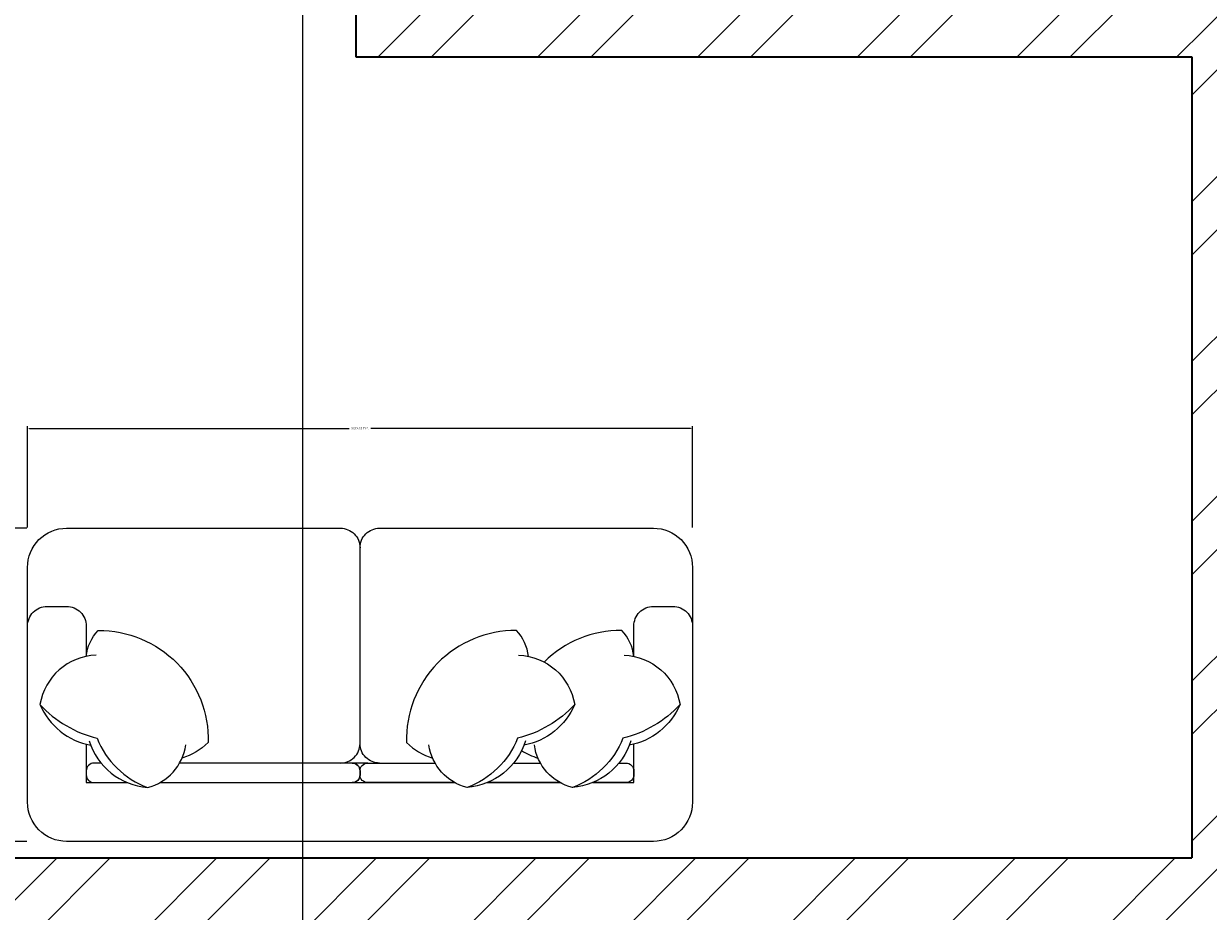
# Model space of a CAD drawing. Units: inches. Extents: x 2552 to 3217, y 1417 to 2737.
# Tile 22 of 25: x 3013 to 3113, y 2392 to 2466. Entities that reach past the tile are written whole.
import ezdxf

# ---------------------------------------------------------------- set-up
doc = ezdxf.new("R2010")
doc.units = ezdxf.units.IN
for name, color, linetype, lineweight in [('A-ANNO-DIMS', 2, 'Continuous', 18), ('A-FURN', 8, 'Continuous', 13), ('A-WALL', 7, 'Continuous', 35), ('A-WALL-PATT', 217, 'Continuous', 13)]:
    doc.layers.add(name, color=color, linetype=linetype, lineweight=lineweight)
doc.styles.get("Standard").update_dxf_attribs({"font": 'arial.ttf'})
doc.dimstyles.get("Standard").update_dxf_attribs({"dimtxt": 0.18, "dimasz": 0.18, "dimexe": 0.18, "dimexo": 0.0625, "dimgap": 0.09, "dimtad": 0, "dimtih": 1, "dimtoh": 1, "dimdec": 4, "dimzin": 0, "dimdsep": 46, "dimtxsty": 'Standard', "dimcen": 0.09, "dimadec": 0, "dimazin": 0, "dimtfac": 1, "dimtdec": 4, "dimtofl": 0, "dimtmove": 0, "dimatfit": 3, "dimfxl": 1, "dimtolj": 1, "dimtzin": 0, "dimarcsym": 0})

# ---------------------------------------------------------------- blocks, each defined once
blk = doc.blocks.new('SOFA-WIDE')
at = {"ltscale": 0.03}
blk.add_lwpolyline([(26.393, 26.393, -0.414214), (28.042, 24.744, -0.414214), (29.692, 26.393), (52.786, 26.393, -0.414214), (56.085, 23.094), (56.085, 3.299, -0.414214), (52.786, 0), (3.299, 0, -0.414214), (0, 3.299), (0, 23.094, -0.414214), (3.299, 26.393), (26.393, 26.393, -0.414214), (28.042, 24.744, -0.414214), (29.692, 26.393)], format="xyb", dxfattribs=at)
for points in [[(26.393, 6.599, 0.414214), (28.042, 8.248), (28.042, 24.744, 0.414214)], [(29.692, 6.599, -0.414214), (28.042, 8.248), (28.042, 24.744, -0.414214)], [(0, 18.146, -0.414214), (1.649, 19.795), (3.299, 19.795, -0.414214), (4.949, 18.146), (4.949, 15.59)], [(51.136, 15.59), (51.136, 18.146, -0.414214), (52.786, 19.795), (54.435, 19.795, -0.414214), (56.085, 18.146)], [(4.945, 15.589, -0.165541), (5.965, 17.769, -0.425989), (15.23, 8.319, -0.121523), (13.031, 7.016, 7.115464)], [(42.254, 15.589, 0.165541), (41.233, 17.769, 0.425989), (31.969, 8.319, 0.121523), (34.168, 7.016, -7.115464)], [(51.14, 15.589, 0.165541), (50.119, 17.769, 0.200231), (43.571, 15.114, 0.121523)], [(5.776, 15.69, 0.356772), (1.05, 11.532, 0.249542), (5.332, 8.105, -9.61688)], [(41.422, 15.69, -0.356772), (46.149, 11.532, -0.249542), (41.866, 8.105, 9.61688)], [(50.308, 15.69, -0.356772), (55.035, 11.532, -0.249542), (50.752, 8.105, 9.61688)], [(1.05, 11.532, 0.14773), (5.871, 8.697, 0.213343), (10.125, 4.539, 0.178662)], [(46.149, 11.532, -0.14773), (41.328, 8.697, -0.213343), (37.074, 4.539, -0.178662)], [(55.035, 11.532, -0.14773), (50.214, 8.697, -0.213343), (45.96, 4.539, -0.178662)], [(5.205, 8.471, 0.306663), (10.125, 4.539, 0.30633), (13.339, 8.13, -0.872847)], [(26.393, 6.599, 0.414214), (28.042, 8.248)], [(29.692, 6.599, -0.414214), (28.042, 8.248)], [(41.994, 8.471, -0.306663), (37.074, 4.539, -0.30633), (33.86, 8.13, 0.872847)], [(50.88, 8.471, -0.306663), (45.96, 4.539, -0.30633), (42.746, 8.13, 0.872847)], [(47.666, 4.949), (51.136, 4.949), (51.136, 8.191, -0.414214)], [(41.671, 7.661, 0.071865), (43.054, 7.016, -7.115464)], [(6.207, 6.599), (5.608, 6.599, 0.414214), (4.949, 5.939), (4.949, 5.609, 0.414214), (5.608, 4.949)], [(11.163, 4.949), (27.383, 4.949, 0.414214), (28.042, 5.609), (28.042, 5.939, 0.414214), (27.383, 6.599), (12.824, 6.599, 0.414214)], [(36.036, 4.949), (28.702, 4.949, -0.414214), (28.042, 5.609), (28.042, 5.939, -0.414214), (28.702, 6.599), (34.375, 6.599, -0.414214)], [(40.991, 6.599), (43.261, 6.599, -0.414214)], [(49.877, 6.599), (50.476, 6.599, -0.414214), (51.136, 5.939), (51.136, 5.609, -0.414214), (50.476, 4.949)], [(5.608, 4.949), (8.419, 4.949, 0.414214)], [(44.922, 4.949), (38.78, 4.949, -0.414214)], [(50.476, 4.949), (47.666, 4.949, -0.414214)]]:
    blk.add_lwpolyline(points, format="xyb")
for points in [[(4.949, 8.191), (4.949, 4.949), (8.419, 4.949)], [(11.163, 4.949), (36.036, 4.949)], [(38.78, 4.949), (44.922, 4.949)]]:
    blk.add_lwpolyline(points)
blk.add_lwpolyline([(27.383, 4.949), (28.702, 4.949, -0.414214), (28.042, 5.609), (28.042, 5.939, -0.414214), (28.702, 6.599), (27.383, 6.599, -0.414214), (28.042, 5.939), (28.042, 5.609, -0.414214)], format="xyb", close=True)
blk = doc.blocks.new('*D45')
at = {"layer": 'A-ANNO-DIMS', "color": 0, "lineweight": -2, "transparency": 16777216}
for p, q in [((3013.159, 2423.861), (3013.159, 2432.391)), ((3013.339, 2432.211), (3040.296, 2432.211)), ((3069.064, 2432.211), (3042.106, 2432.211)), ((3069.244, 2423.861), (3069.244, 2432.391))]:
    blk.add_line(p, q, dxfattribs=at)
at = {"layer": 'A-ANNO-DIMS', "color": 0, "transparency": 16777216}
for points in [[(3013.339, 2432.241), (3013.339, 2432.181), (3013.159, 2432.211)], [(3069.064, 2432.241), (3069.064, 2432.181), (3069.244, 2432.211)]]:
    blk.add_solid(points, dxfattribs=at)
at = {"layer": 'Defpoints', "color": 0, "transparency": 16777216}
for p in [(3069.244, 2432.211), (3013.159, 2423.798), (3069.244, 2423.798)]:
    blk.add_point(p, dxfattribs=at)
at = {"layer": 'A-ANNO-DIMS', "color": 0, "transparency": 16777216, "insert": (3041.201, 2432.211), "char_height": 0.18, "attachment_point": 5}
blk.add_mtext('\\A1;SOFA 56 TYP.', dxfattribs=at)
blk = doc.blocks.new('*D46')
at = {"layer": 'A-ANNO-DIMS', "color": 0, "lineweight": -2, "transparency": 16777216}
for p, q in [((3013.096, 2423.798), (3004.566, 2423.798)), ((3004.746, 2423.618), (3004.746, 2410.784)), ((3004.746, 2397.585), (3004.746, 2410.42)), ((3013.096, 2397.405), (3004.566, 2397.405))]:
    blk.add_line(p, q, dxfattribs=at)
at = {"layer": 'A-ANNO-DIMS', "color": 0, "transparency": 16777216}
for points in [[(3004.716, 2423.618), (3004.776, 2423.618), (3004.746, 2423.798)], [(3004.716, 2397.585), (3004.776, 2397.585), (3004.746, 2397.405)]]:
    blk.add_solid(points, dxfattribs=at)
at = {"layer": 'Defpoints', "color": 0, "transparency": 16777216}
for p in [(3004.746, 2423.798), (3013.159, 2423.798), (3013.159, 2397.405)]:
    blk.add_point(p, dxfattribs=at)
at = {"layer": 'A-ANNO-DIMS', "color": 0, "transparency": 16777216, "insert": (3004.746, 2410.602), "char_height": 0.18, "attachment_point": 5}
blk.add_mtext('\\A1;26 TYP.', dxfattribs=at)
blk = doc.blocks.new('*D57')
at = {"layer": 'A-ANNO-DIMS', "color": 0, "lineweight": -2, "transparency": 16777216}
for p, q in [((3004.084, 2515.95), (3004.084, 1482.533)), ((3036.34, 2515.95), (3036.34, 1482.533)), ((3004.264, 1482.713), (3019.748, 1482.713)), ((3036.16, 1482.713), (3020.676, 1482.713))]:
    blk.add_line(p, q, dxfattribs=at)
at = {"layer": 'A-ANNO-DIMS', "color": 0, "transparency": 16777216}
for points in [[(3004.264, 1482.743), (3004.264, 1482.683), (3004.084, 1482.713)], [(3036.16, 1482.743), (3036.16, 1482.683), (3036.34, 1482.713)]]:
    blk.add_solid(points, dxfattribs=at)
at = {"layer": 'Defpoints', "color": 0, "transparency": 16777216}
for p in [(3004.084, 2516.013), (3036.34, 2516.013), (3036.34, 1482.713)]:
    blk.add_point(p, dxfattribs=at)
at = {"layer": 'A-ANNO-DIMS', "color": 0, "transparency": 16777216, "insert": (3020.212, 1482.713), "char_height": 0.18, "attachment_point": 5}
blk.add_mtext('\\A1;32.255', dxfattribs=at)
blk = doc.blocks.new('*D66')
at = {"layer": 'A-ANNO-DIMS', "color": 0, "lineweight": -2, "transparency": 16777216}
for p, q in [((3120.416, 2481.184), (3180.334, 2481.184)), ((3180.154, 2481.004), (3180.154, 2434.28)), ((3180.154, 2387.193), (3180.154, 2433.916)), ((3111.416, 2387.013), (3180.334, 2387.013))]:
    blk.add_line(p, q, dxfattribs=at)
at = {"layer": 'A-ANNO-DIMS', "color": 0, "transparency": 16777216}
for points in [[(3180.124, 2481.004), (3180.184, 2481.004), (3180.154, 2481.184)], [(3180.124, 2387.193), (3180.184, 2387.193), (3180.154, 2387.013)]]:
    blk.add_solid(points, dxfattribs=at)
at = {"layer": 'Defpoints', "color": 0, "transparency": 16777216}
for p in [(3120.354, 2481.184), (3111.354, 2387.013), (3180.154, 2387.013)]:
    blk.add_point(p, dxfattribs=at)
at = {"layer": 'A-ANNO-DIMS', "color": 0, "transparency": 16777216, "insert": (3180.154, 2434.098), "char_height": 0.18, "attachment_point": 5}
blk.add_mtext('\\A1;94.17', dxfattribs=at)

msp = doc.modelspace()

# ---------------------------------------------------------------- hatches: boundary and pattern name
at = {"layer": 'A-WALL-PATT'}
h = msp.add_hatch(dxfattribs=at)
h.set_pattern_fill('ANSI32', color=256)
h.paths.add_polyline_path([(2756.676, 2649.5125), (2637.3535, 2649.5125), (2637.3535, 2617.9626), (2641.8535, 2617.9626), (2646.3535, 2617.9626), (2646.3535, 2640.5125), (2724.3535, 2640.5125), (2724.3535, 2520.5125), (2720.299, 2520.5125), (2720.299, 2516.0125), (2733.4075, 2516.0125), (2733.4075, 2518.2213), (2733.4075, 2520.5125), (2728.8535, 2520.5125), (2728.8535, 2640.5125), (2756.676, 2640.5125)])
h.paths.add_polyline_path([(2848.8535, 2649.5125), (2804.676, 2649.5125), (2804.676, 2640.5125), (2839.8535, 2640.5125), (2839.8535, 2598.3517), (2848.8535, 2598.3517)])
h.paths.add_polyline_path([(2646.3535, 2516.0125), (2697.9593, 2516.0125), (2697.9593, 2518.2625), (2697.9593, 2520.5125), (2646.3535, 2520.5125), (2646.3535, 2581.9626), (2637.3535, 2581.9626), (2637.3535, 2364.3298), (2646.3535, 2364.3298), (2646.3535, 2387.0125), (2724.3535, 2387.0125), (2724.3535, 2267.0125), (2721.0443, 2267.0125), (2721.0443, 2262.5125), (2733.7854, 2262.5125), (2733.7854, 2264.7625), (2733.7854, 2267.0125), (2728.8535, 2267.0125), (2728.8535, 2387.0125), (2839.8535, 2387.0125), (2839.8535, 2363.8387), (2848.8535, 2363.8387), (2848.8535, 2403.7415), (2844.3535, 2403.7415), (2839.8535, 2403.7415), (2839.8535, 2396.0125), (2646.3535, 2396.0125)])
h.paths.add_polyline_path([(2848.8535, 2550.3517), (2844.3535, 2550.3517), (2839.8535, 2550.3517), (2839.8535, 2520.5125), (2801.9195, 2520.5125), (2801.9195, 2518.2625), (2801.9195, 2516.0125), (2839.8535, 2516.0125), (2839.8535, 2507.5813), (2848.8535, 2507.5813)], flags=17)
h.paths.add_polyline_path([(2848.8535, 2483.5813), (2844.3535, 2483.5813), (2839.8535, 2483.5813), (2839.8535, 2468.0125), (2773.8535, 2468.0125), (2773.8535, 2516.0125), (2778.1336, 2516.0125), (2778.1336, 2520.5125), (2766.696, 2520.5125), (2766.696, 2518.2625), (2766.696, 2516.0125), (2769.3535, 2516.0125), (2769.3535, 2463.5125), (2839.8535, 2463.5125), (2839.8535, 2431.0782), (2848.8535, 2431.0782)], flags=17)
h.paths.add_polyline_path([(2917.8535, 2569.2764), (2913.3535, 2569.2764), (2908.8535, 2569.2764), (2908.8535, 2433.001), (2917.8535, 2433.001), (2917.8535, 2516.0125), (2967.486, 2516.0125), (2967.486, 2520.5125), (2917.8535, 2520.5125)])
h.paths.add_polyline_path([(3000.3535, 2640.5125), (2995.8535, 2640.5125), (2995.8535, 2520.5125), (2990.688, 2520.5125), (2990.688, 2516.0125), (3004.0844, 2516.0125), (3004.0844, 2518.2625), (3004.0844, 2520.5125), (3000.3535, 2520.5125)])
h.paths.add_polyline_path([(3120.3535, 2561.3689), (3115.8535, 2561.3689), (3111.3535, 2561.3689), (3111.3535, 2520.5125), (3070.9814, 2520.5125), (3070.9814, 2518.2625), (3070.9814, 2516.0125), (3111.3535, 2516.0125), (3111.3535, 2505.1841), (3120.3535, 2505.1841)])
h.paths.add_polyline_path([(3120.3535, 2481.1841), (3115.8535, 2481.1841), (3111.3535, 2481.1841), (3111.3535, 2468.0125), (3045.3535, 2468.0125), (3045.3535, 2516.0125), (3048.9787, 2516.0125), (3048.9787, 2520.5125), (3036.3395, 2520.5125), (3036.3395, 2516.0125), (3040.8535, 2516.0125), (3040.8535, 2463.5125), (3111.3535, 2463.5125), (3111.3535, 2396.0125), (2917.8535, 2396.0125), (2917.8535, 2403.4124), (2913.3535, 2403.4124), (2908.8535, 2403.4124), (2908.8535, 2182.5756), (2917.8535, 2182.5756), (2917.8535, 2262.5125), (2968.001, 2262.5125), (2968.001, 2264.7625), (2968.001, 2267.0125), (2917.8535, 2267.0125), (2917.8535, 2387.0125), (3111.3535, 2387.0125), (3111.3535, 2352.2435), (3120.3535, 2352.2435)])
h.paths.add_polyline_path([(3120.3535, 2304.2435), (3115.8535, 2304.2435), (3111.3535, 2304.2435), (3111.3535, 2267.0125), (3073.8616, 2267.0125), (3073.8616, 2264.7625), (3073.8616, 2262.5125), (3111.3535, 2262.5125), (3111.3535, 2252.376), (3120.3535, 2252.376)], flags=17)
h.paths.add_polyline_path([(3120.3535, 2228.376), (3115.8535, 2228.376), (3111.3535, 2228.376), (3111.3535, 2214.5125), (3045.3535, 2214.5125), (3045.3535, 2262.5125), (3049.3096, 2262.5125), (3049.3096, 2267.0125), (3035.0125, 2267.0125), (3035.0125, 2262.5125), (3040.8535, 2262.5125), (3040.8535, 2210.0125), (3111.3535, 2210.0125), (3111.3535, 2142.5125), (2917.8535, 2142.5125), (2917.8535, 2150.2408), (2913.3535, 2150.2408), (2908.8535, 2150.2408), (2908.8535, 1924.9905), (2917.8535, 1924.9905), (2917.8535, 2009.0125), (2971.959, 2009.0125), (2971.959, 2011.2625), (2971.959, 2013.5125), (2917.8535, 2013.5125), (2917.8535, 2133.5125), (2995.8535, 2133.5125), (2995.8535, 2013.5125), (2992.1797, 2013.5125), (2992.1797, 2009.0125), (3004.3344, 2009.0125), (3004.3344, 2011.2625), (3004.3344, 2013.5125), (3000.3535, 2013.5125), (3000.3535, 2133.5125), (3111.3535, 2133.5125), (3111.3535, 2115.0291), (3120.3535, 2115.0291)])
h.paths.add_polyline_path([(3000.3535, 2387.0125), (2995.8535, 2387.0125), (2995.8535, 2267.0125), (2991.3326, 2267.0125), (2991.3326, 2262.5125), (3004.1044, 2262.5125), (3004.1044, 2264.7625), (3004.1044, 2267.0125), (3000.3535, 2267.0125)], flags=17)
h.paths.add_polyline_path([(3120.3535, 1973.2388), (3115.8535, 1973.2388), (3111.3535, 1973.2388), (3111.3535, 1961.0125), (3045.3535, 1961.0125), (3045.3535, 2009.0125), (3048.9101, 2009.0125), (3048.9101, 2013.5125), (3037.105, 2013.5125), (3037.105, 2011.2625), (3037.105, 2009.0125), (3040.8535, 2009.0125), (3040.8535, 1956.5125), (3111.3535, 1956.5125), (3111.3535, 1889.0125), (2917.8535, 1889.0125), (2917.8535, 1895.7215), (2913.3535, 1895.7215), (2908.8535, 1895.7215), (2908.8535, 1844.2217), (2917.8535, 1844.2217), (2917.8535, 1880.0125), (3111.3535, 1880.0125), (3111.3535, 1846.9541), (3120.3535, 1846.9541)])
h.paths.add_polyline_path([(3120.3535, 2067.0291), (3111.3535, 2067.0291), (3111.3535, 2013.5125), (3071.3001, 2013.5125), (3071.3001, 2009.0125), (3111.3535, 2009.0125), (3111.3535, 1997.2388), (3120.3535, 1997.2388)], flags=0)
h.paths.add_polyline_path([(3120.3535, 1798.9541), (3115.8535, 1798.9541), (3111.3535, 1798.9541), (3111.3535, 1760.0125), (3071.2497, 1760.0125), (3071.2497, 1757.7625), (3071.2497, 1755.5125), (3111.3535, 1755.5125), (3111.3535, 1746.162), (3120.3535, 1746.2478)])
h.paths.add_polyline_path([(3120.3535, 1722.2049), (3111.3535, 1722.2049), (3111.3535, 1707.5125), (3045.3535, 1707.5125), (3045.3535, 1755.5125), (3048.6624, 1755.5125), (3048.6624, 1760.0125), (3035.3703, 1760.0125), (3035.3703, 1755.5125), (3040.8535, 1755.5125), (3040.8535, 1703.0125), (3111.3535, 1703.0125), (3111.3535, 1635.5125), (2917.8535, 1635.5125), (2917.8535, 1643.1366), (2913.3535, 1643.1366), (2908.8535, 1643.1366), (2908.8535, 1626.5125), (3120.3535, 1626.5125)])
h.paths.add_polyline_path([(2917.8535, 1755.5125), (2973.2287, 1755.5125), (2973.2287, 1757.7625), (2973.2287, 1760.0125), (2917.8535, 1760.0125), (2917.8535, 1808.2217), (2913.3535, 1808.2217), (2908.8535, 1808.2217), (2908.8535, 1676.1665), (2917.8535, 1676.1665)])
h.paths.add_polyline_path([(3000.3535, 1880.0125), (2995.8535, 1880.0125), (2995.8535, 1760.0125), (2992.9329, 1760.0125), (2992.9329, 1755.5125), (3003.8766, 1755.5125), (3003.8766, 1757.7625), (3003.8766, 1760.0125), (3000.3535, 1760.0125)])
h.paths.add_polyline_path([(2848.8535, 1896.6971), (2844.3535, 1896.6971), (2839.8535, 1896.6971), (2839.8535, 1889.0125), (2646.3535, 1889.0125), (2646.3535, 2009.0125), (2700.5253, 2009.0125), (2700.5253, 2011.2625), (2700.5253, 2013.5125), (2646.3535, 2013.5125), (2646.3535, 2053.1812), (2641.8535, 2053.1812), (2637.3535, 2053.1812), (2637.3535, 1836.254), (2646.3535, 1836.254), (2646.3535, 1880.0125), (2724.3535, 1880.0125), (2724.3535, 1760.0125), (2721.2473, 1760.0125), (2721.2473, 1755.5125), (2731.9187, 1755.5125), (2731.9187, 1757.7625), (2731.9187, 1760.0125), (2728.8535, 1760.0125), (2728.8535, 1880.0125), (2839.8535, 1880.0125), (2839.8535, 1840.3813), (2848.8535, 1840.3813)])
h.paths.add_polyline_path([(2848.8535, 1792.3813), (2844.3535, 1792.3813), (2839.8535, 1792.3813), (2839.8535, 1760.0125), (2797.8845, 1760.0125), (2797.8845, 1755.5125), (2839.8535, 1755.5125), (2839.8535, 1743.3688), (2844.3535, 1743.3688), (2848.8535, 1743.3688)], flags=0)
h.paths.add_polyline_path([(2848.8535, 1719.3688), (2844.3535, 1719.3688), (2839.8535, 1719.3688), (2839.8535, 1707.5125), (2773.8535, 1707.5125), (2773.8535, 1755.5125), (2777.716, 1755.5125), (2777.716, 1760.0125), (2760.9247, 1760.0125), (2760.9247, 1757.9721), (2760.9247, 1755.5125), (2769.3535, 1755.5125), (2769.3535, 1703.0125), (2839.8535, 1703.0125), (2839.8535, 1673.0277), (2848.8535, 1672.9407)], flags=0)
h.paths.add_polyline_path([(2646.3535, 1755.5125), (2702.9171, 1755.5125), (2702.9171, 1757.7625), (2702.9171, 1760.0125), (2646.3535, 1760.0125), (2646.3535, 1800.254), (2641.8535, 1800.254), (2637.3535, 1800.254), (2637.3535, 1626.5125), (2848.8535, 1626.5125), (2848.8535, 1643.1187), (2844.3535, 1643.1187), (2839.8535, 1643.1187), (2839.8535, 1635.5125), (2646.3535, 1635.5125)])
h.paths.add_polyline_path([(2848.8535, 2148.8427), (2844.3535, 2148.8427), (2839.8535, 2148.8427), (2839.8535, 2142.5125), (2646.3535, 2142.5125), (2646.3535, 2262.5125), (2701.3562, 2262.5125), (2701.3562, 2264.7625), (2701.3562, 2267.0125), (2646.3535, 2267.0125), (2646.3535, 2328.3298), (2637.3535, 2328.3298), (2637.3535, 2089.1812), (2646.3535, 2089.1812), (2646.3535, 2133.5125), (2839.8535, 2133.5125), (2839.8535, 2097.5966), (2848.8535, 2097.5966)])
h.paths.add_polyline_path([(2728.8535, 2133.5125), (2724.3535, 2133.5125), (2724.3535, 2013.5125), (2719.6039, 2013.5125), (2719.6039, 2009.0125), (2732.5784, 2009.0125), (2732.5784, 2011.2625), (2732.5784, 2013.5125), (2728.8535, 2013.5125)])
h.paths.add_polyline_path([(2848.8535, 1970.0557), (2844.3535, 1970.0557), (2839.8535, 1970.0557), (2839.8535, 1961.0125), (2773.8535, 1961.0125), (2773.8535, 2009.0125), (2777.3388, 2009.0125), (2777.3388, 2013.5125), (2764.7681, 2013.5125), (2764.7681, 2009.0125), (2769.3535, 2009.0125), (2769.3535, 1956.5125), (2839.8535, 1956.5125), (2839.8535, 1924.7199), (2848.8535, 1924.7199)], flags=17)
h.paths.add_polyline_path([(2848.8535, 2049.5966), (2844.3535, 2049.5966), (2839.8535, 2049.5966), (2839.8535, 2013.5125), (2798.198, 2013.5125), (2798.198, 2011.2625), (2798.198, 2009.0125), (2839.8535, 2009.0125), (2839.8535, 1994.0557), (2848.8535, 1994.0557)], flags=17)
h.paths.add_polyline_path([(2848.8535, 2315.8387), (2839.8535, 2315.8387), (2839.8535, 2267.0125), (2799.3375, 2267.0125), (2799.3375, 2264.7625), (2799.3375, 2262.5125), (2839.8535, 2262.5125), (2839.8535, 2253.2843), (2848.8535, 2253.2843)], flags=17)
h.paths.add_polyline_path([(2848.8535, 2229.2843), (2839.8535, 2229.2843), (2839.8535, 2177.6936), (2848.8535, 2177.6936)], flags=17)
h.paths.add_polyline_path([(2839.8535, 2214.5125), (2773.8535, 2214.5125), (2773.8535, 2262.5125), (2777.6984, 2262.5125), (2777.6984, 2267.0125), (2763.8226, 2267.0125), (2763.8226, 2262.5125), (2769.3535, 2262.5125), (2769.3535, 2210.0125), (2839.8535, 2210.0125)], flags=17)
h.paths.add_polyline_path([(3050.32, 2520.2817), (3088.9114, 2520.2817), (3088.9114, 2538.939), (3050.32, 2538.939)], flags=9)

# ---------------------------------------------------------------- linework, layer by layer
at = {"layer": 'A-WALL'}
for p, q in [((3040.8535, 2516.0125), (3040.8535, 2463.5125)), ((3040.8535, 2463.5125), (3111.3535, 2463.5125)), ((3111.3535, 2463.5125), (3111.3535, 2396.0125)), ((2917.8535, 2396.0125), (3111.3535, 2396.0125))]:
    msp.add_line(p, q, dxfattribs=at)

# ---------------------------------------------------------------- block references
at = {"layer": 'A-FURN'}
msp.add_blockref('SOFA-WIDE', (3013.159, 2397.405), dxfattribs=at)

# ---------------------------------------------------------------- dimensions: what is measured, and where the dimension line sits
at = {"layer": 'A-ANNO-DIMS'}
dim = msp.add_linear_dim(base=(3036.3395, 1482.7125), p1=(3004.0844, 2516.0125), p2=(3036.3395, 2516.0125), dimstyle='Standard', override={"dimdec": 3, "dimlfac": 1, "dimrnd": 0, "dimzin": 0, "dimdsep": 46, "dimlunit": 2}, dxfattribs=at)
dim.commit()
dim.dimension.update_dxf_attribs({"geometry": '*D57', "text_midpoint": (3020.212, 1482.7125)})
dim = msp.add_linear_dim(base=(3180.1535, 2387.0125), p1=(3120.3535, 2481.1841), p2=(3111.3535, 2387.0125), angle=90, dimstyle='Standard', override={"dimdec": 2, "dimlfac": 1, "dimrnd": 0, "dimzin": 0, "dimdsep": 46, "dimlunit": 2}, dxfattribs=at)
dim.commit()
dim.dimension.update_dxf_attribs({"geometry": '*D66', "text_midpoint": (3180.1535, 2434.0983)})
dim = msp.add_linear_dim(base=(3069.244, 2432.2111), p1=(3013.1588, 2423.7983), p2=(3069.244, 2423.7983), text='SOFA <> TYP.', dimstyle='Standard', override={"dimdec": 0, "dimlfac": 1, "dimrnd": 0, "dimzin": 0, "dimdsep": 46, "dimlunit": 2}, dxfattribs=at)
dim.commit()
dim.dimension.update_dxf_attribs({"geometry": '*D45', "text_midpoint": (3041.2014, 2432.2111)})
dim = msp.add_linear_dim(base=(3004.746, 2423.7983), p1=(3013.1588, 2397.4053), p2=(3013.1588, 2423.7983), angle=90, text='<> TYP.', dimstyle='Standard', override={"dimdec": 0, "dimlfac": 1, "dimrnd": 0, "dimzin": 0, "dimdsep": 46, "dimlunit": 2}, dxfattribs=at)
dim.commit()
dim.dimension.update_dxf_attribs({"geometry": '*D46', "text_midpoint": (3004.746, 2410.6018)})

doc.saveas('drawing.dxf')
